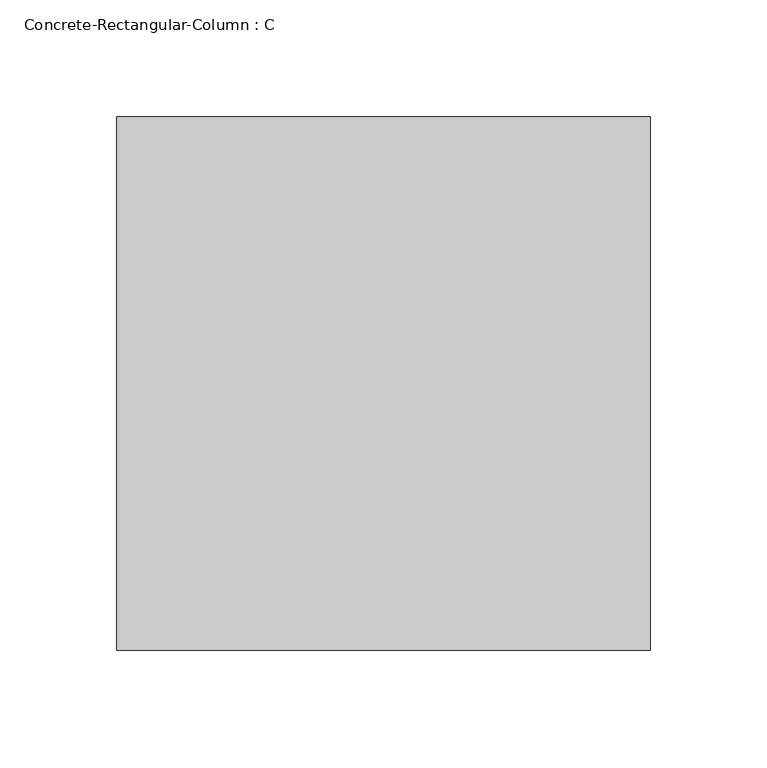
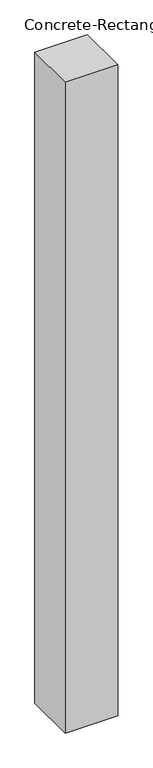
"""IFC4 building model written with IfcOpenShell, lengths in millimetres: column geometry, Concrete-Rectangular-Column : C."""

from ifc_helpers import new_model, si_unit, origin, origin_with_axes, place, context, project, spatial, polyline, outline, extrude, source, transform, mapped, element, save


def concrete_rectangular_column_c_80bd43f1(model_context):
    return source(origin(), model_context, "Body", "SweptSolid", [
        extrude(outline(polyline([(114.3, 114.3), (114.3, -114.3), (-114.3, -114.3), (-114.3, 114.3), (114.3, 114.3)])), origin_with_axes(), (0.0, 0.0, 1.0), 3000.0),
    ])


if __name__ == "__main__":
    model = new_model("IFC4")
    model_context = context("Model", 3, world=origin())
    ifc_project = project(units=[si_unit("LENGTHUNIT", "METRE", prefix="MILLI")], contexts=[model_context])
    site = spatial("IfcSite", under=ifc_project)
    building = spatial("IfcBuilding", under=site)
    placement = place(None, origin())
    concrete_rectangular_column_c_shape = concrete_rectangular_column_c_80bd43f1(model_context)
    element("IfcColumn", 1, ObjectType="Concrete-Rectangular-Column : C", at=placement, inside=building, context=model_context, shape_type="MappedRepresentation", body=[
        mapped(concrete_rectangular_column_c_shape, transform((0.0, 0.0, 0.0), x_axis=(1.0, 0.0, 0.0), y_axis=(0.0, 1.0, 0.0), z_axis=(0.0, 0.0, 1.0))),
    ])
    save(model, "model.ifc")

# Revit data of these elements
# Type "Concrete-Rectangular-Column : C"
#   b = 228.6 mm
#   h = 228.6 mm
#   Structural Material [instance default] = Concrete, Cast-in-Place gray
# Element 1 (IfcColumn, "Concrete-Rectangular-Column : C")
#   Materials on its faces: "Concrete, Cast-in-Place gray"
# Materials
#   "Concrete, Cast-in-Place gray": class "Concrete", colour RGB 192 192 192, transparency 0, Description = "Cast-in-place concrete", Cost = 0
